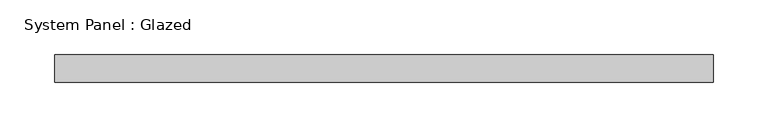
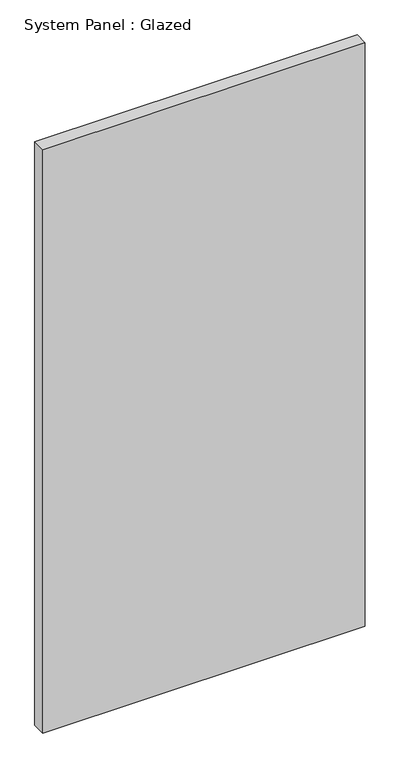
"""IFC4 building model written with IfcOpenShell, lengths in millimetres: plate geometry, System Panel : Glazed."""

from ifc_helpers import new_model, si_unit, origin, origin_with_axes, place, context, project, spatial, polyline, outline, extrude, source, transform, mapped, element, save


def system_panel_glazed_7487696a(model_context):
    return source(origin(), model_context, "Body", "SweptSolid", [
        extrude(outline(polyline([(302.2204434, 19.05), (-302.2204434, 19.05), (-302.2204434, 44.45), (302.2204434, 44.45), (302.2204434, 19.05)])), origin_with_axes(), (0.0, 0.0, 1.0), 1155.7),
    ])


if __name__ == "__main__":
    model = new_model("IFC4")
    model_context = context("Model", 3, world=origin())
    ifc_project = project(units=[si_unit("LENGTHUNIT", "METRE", prefix="MILLI")], contexts=[model_context])
    site = spatial("IfcSite", under=ifc_project)
    building = spatial("IfcBuilding", under=site)
    placement = place(None, origin())
    system_panel_glazed_shape = system_panel_glazed_7487696a(model_context)
    element("IfcPlate", 1, ObjectType="System Panel : Glazed", at=placement, inside=building, context=model_context, shape_type="MappedRepresentation", body=[
        mapped(system_panel_glazed_shape, transform((0.0, 0.0, 0.0), x_axis=(1.0, 0.0, 0.0), y_axis=(0.0, 1.0, 0.0), z_axis=(0.0, 0.0, 1.0))),
    ])
    save(model, "model.ifc")

# Revit data of these elements
# Type "System Panel : Glazed"
#   Construction Type Id = "GSP4R"
#   Analytic Construction = "1/8 in Pilkington single glazing"
#   Visual Light Transmittance = 0.9
#   Solar Heat Gain Coefficient = 0.86
#   Heat Transfer Coefficient (U) = 1.18115 BTU/(h·ft²·°F)
# Element 1 (IfcPlate, "System Panel : Glazed")
#   Materials on its faces: "Glass"
# Materials
#   "Glass": class "Glass", colour RGB 0 128 192, transparency 0.75, Description = "Soda Lime Glass", Cost = 0
